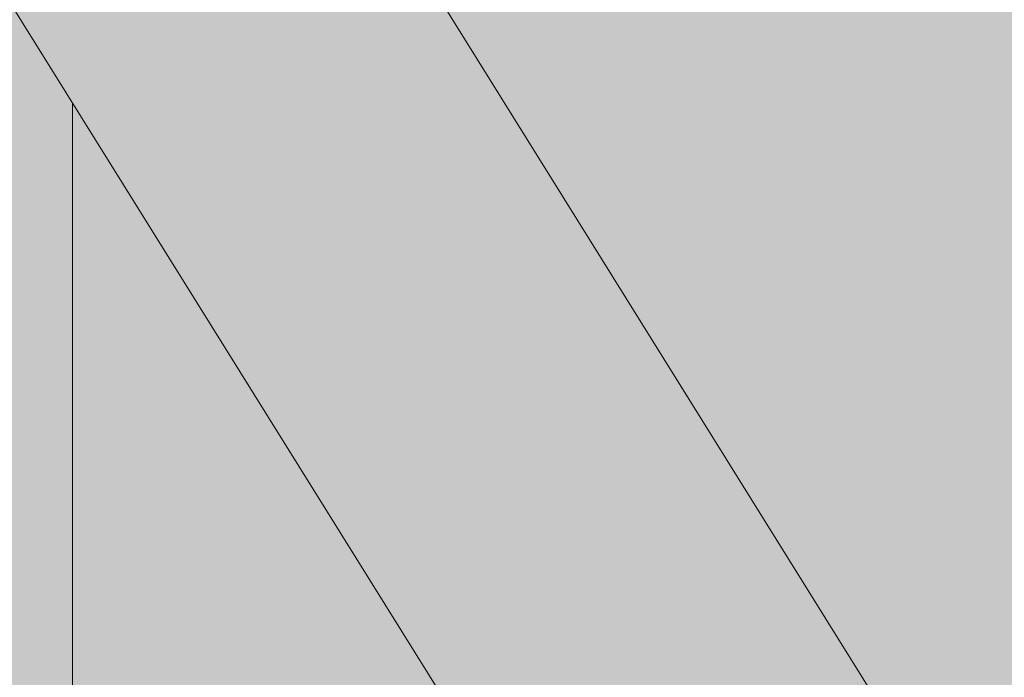
# Model space of a CAD drawing. Units: millimetres. Extents: x 11032 to 26788, y 3406 to 24505.
# Tile 50 of 78: x 15652 to 15786, y 16276 to 16366. Entities that reach past the tile are written whole.
import ezdxf

# ---------------------------------------------------------------- set-up
doc = ezdxf.new("R2010")
doc.units = ezdxf.units.MM
doc.header["$MEASUREMENT"] = 0
for name, color, linetype, lineweight in [('A-ANNO-DIMS', 2, 'Continuous', 18), ('A-GLAZ', 250, 'Continuous', 20), ('A-ROOF', 7, 'Continuous', 30), ('A-WALL', 7, 'Continuous', 35), ('E-LITE', 7, 'Continuous', 18), ('E-LITE-PATT', 7, 'Continuous', 13)]:
    doc.layers.add(name, color=color, linetype=linetype, lineweight=lineweight)
for name, color, linetype, lineweight, true_color in [('A-GLAZ-FRAM-PATT', 250, 'Continuous', 13, 0x262627), ('A-ROOF-PATT', 9, 'Continuous', 13, 0xc7c8ca), ('A-WALL-INTR-PATT', 251, 'Continuous', 13, 0x6c6b6a)]:
    doc.layers.add(name, color=color, linetype=linetype, lineweight=lineweight, true_color=true_color)
doc.styles.get("Standard").update_dxf_attribs({"font": 'arial.ttf'})
doc.dimstyles.get("Standard").update_dxf_attribs({"dimtxt": 150, "dimasz": 100, "dimexe": 10, "dimexo": 5, "dimgap": 5, "dimtad": 0, "dimtih": 1, "dimtoh": 1, "dimdec": 0, "dimzin": 0, "dimdsep": 46, "dimtxsty": 'Standard', "dimcen": 0.09, "dimadec": 0, "dimazin": 0, "dimtfac": 1, "dimtdec": 0, "dimtofl": 0, "dimtmove": 0, "dimatfit": 3, "dimfxl": 1, "dimtolj": 1, "dimtzin": 0, "dimarcsym": 0})

# ---------------------------------------------------------------- blocks, each defined once
blk = doc.blocks.new('*D36')
at = {"layer": 'A-ANNO-DIMS', "color": 0, "lineweight": -2, "transparency": 16777216}
for p, q in [((12301.26, 17115.89), (12301.26, 24416.86)), ((25397.4, 4466.4), (25397.4, 24416.86)), ((12401.26, 24406.86), (18569.2, 24406.86)), ((25297.4, 24406.86), (19129.47, 24406.86))]:
    blk.add_line(p, q, dxfattribs=at)
at = {"layer": 'A-ANNO-DIMS', "color": 0, "transparency": 16777216}
for points in [[(12401.26, 24423.52), (12401.26, 24390.19), (12301.26, 24406.86)], [(25297.4, 24423.52), (25297.4, 24390.19), (25397.4, 24406.86)]]:
    blk.add_solid(points, dxfattribs=at)
at = {"layer": 'Defpoints', "color": 0, "transparency": 16777216}
for p in [(25397.4, 24406.86), (12301.26, 17110.89), (25397.4, 4461.4)]:
    blk.add_point(p, dxfattribs=at)
at = {"layer": 'A-ANNO-DIMS', "color": 0, "transparency": 16777216, "insert": (18849.33, 24406.86), "char_height": 150, "attachment_point": 5}
blk.add_mtext('\\A1;13096', dxfattribs=at)
blk = doc.blocks.new('*D37')
at = {"layer": 'A-ANNO-DIMS', "color": 0, "lineweight": -2, "transparency": 16777216}
for p, q in [((18087.74, 23450.36), (11334.76, 23450.36)), ((11344.76, 23350.36), (11344.76, 14037.46)), ((11344.76, 4561.4), (11344.76, 13874.29)), ((12927.66, 4461.4), (11334.76, 4461.4))]:
    blk.add_line(p, q, dxfattribs=at)
at = {"layer": 'A-ANNO-DIMS', "color": 0, "transparency": 16777216}
for points in [[(11328.1, 23350.36), (11361.43, 23350.36), (11344.76, 23450.36)], [(11328.1, 4561.4), (11361.43, 4561.4), (11344.76, 4461.4)]]:
    blk.add_solid(points, dxfattribs=at)
at = {"layer": 'Defpoints', "color": 0, "transparency": 16777216}
for p in [(11344.76, 23450.36), (18092.74, 23450.36), (12932.66, 4461.4)]:
    blk.add_point(p, dxfattribs=at)
at = {"layer": 'A-ANNO-DIMS', "color": 0, "transparency": 16777216, "insert": (11344.76, 13955.88), "char_height": 150, "attachment_point": 5}
blk.add_mtext('\\A1;18989', dxfattribs=at)
blk = doc.blocks.new('*D45')
at = {"layer": 'A-ANNO-DIMS', "color": 0, "lineweight": -2, "transparency": 16777216}
for p, q in [((13792.37, 18518.92), (26363.9, 18518.92)), ((26353.9, 18418.92), (26353.9, 17450.32)), ((26353.9, 16318.44), (26353.9, 17287.05)), ((22902.4, 16218.44), (26363.9, 16218.44))]:
    blk.add_line(p, q, dxfattribs=at)
at = {"layer": 'A-ANNO-DIMS', "color": 0, "transparency": 16777216}
for points in [[(26337.24, 18418.92), (26370.57, 18418.92), (26353.9, 18518.92)], [(26337.24, 16318.44), (26370.57, 16318.44), (26353.9, 16218.44)]]:
    blk.add_solid(points, dxfattribs=at)
at = {"layer": 'Defpoints', "color": 0, "transparency": 16777216}
for p in [(13787.37, 18518.92), (26353.9, 18518.92), (22897.4, 16218.44)]:
    blk.add_point(p, dxfattribs=at)
at = {"layer": 'A-ANNO-DIMS', "color": 0, "transparency": 16777216, "insert": (26353.9, 17368.68), "char_height": 150, "attachment_point": 5}
blk.add_mtext('\\A1;2300.5', dxfattribs=at)
blk = doc.blocks.new('*D57')
at = {"layer": 'A-ANNO-DIMS', "color": 0, "lineweight": -2, "transparency": 16777216}
for p, q in [((14994.7, 7266.4), (14994.7, 24416.86)), ((20894.7, 7266.4), (20894.7, 24416.86)), ((15094.7, 24406.86), (17715.98, 24406.86)), ((20794.7, 24406.86), (18173.42, 24406.86))]:
    blk.add_line(p, q, dxfattribs=at)
at = {"layer": 'A-ANNO-DIMS', "color": 0, "transparency": 16777216}
for points in [[(15094.7, 24423.52), (15094.7, 24390.19), (14994.7, 24406.86)], [(20794.7, 24423.52), (20794.7, 24390.19), (20894.7, 24406.86)]]:
    blk.add_solid(points, dxfattribs=at)
at = {"layer": 'Defpoints', "color": 0, "transparency": 16777216}
for p in [(20894.7, 24406.86), (14994.7, 7261.4), (20894.7, 7261.4)]:
    blk.add_point(p, dxfattribs=at)
at = {"layer": 'A-ANNO-DIMS', "color": 0, "transparency": 16777216, "insert": (17944.7, 24406.86), "char_height": 150, "attachment_point": 5}
blk.add_mtext('\\A1;5900', dxfattribs=at)
blk = doc.blocks.new('*D60')
at = {"layer": 'A-ANNO-DIMS', "color": 0, "lineweight": -2, "transparency": 16777216}
for p, q in [((14994.7, 7266.4), (14994.7, 24416.86)), ((16344.7, 7266.4), (16344.7, 24416.86)), ((15094.7, 24406.86), (15448.04, 24406.86)), ((16244.7, 24406.86), (15891.36, 24406.86))]:
    blk.add_line(p, q, dxfattribs=at)
at = {"layer": 'A-ANNO-DIMS', "color": 0, "transparency": 16777216}
for points in [[(15094.7, 24423.52), (15094.7, 24390.19), (14994.7, 24406.86)], [(16244.7, 24423.52), (16244.7, 24390.19), (16344.7, 24406.86)]]:
    blk.add_solid(points, dxfattribs=at)
at = {"layer": 'Defpoints', "color": 0, "transparency": 16777216}
for p in [(16344.7, 24406.86), (14994.7, 7261.4), (16344.7, 7261.4)]:
    blk.add_point(p, dxfattribs=at)
at = {"layer": 'A-ANNO-DIMS', "color": 0, "transparency": 16777216, "insert": (15669.7, 24406.86), "char_height": 150, "attachment_point": 5}
blk.add_mtext('\\A1;1350', dxfattribs=at)

msp = doc.modelspace()

# ---------------------------------------------------------------- hatches: boundary and pattern name
at = {"layer": 'A-GLAZ-FRAM-PATT'}
h = msp.add_hatch(color=256, dxfattribs=at)
edge = h.paths.add_edge_path()
edge.add_line((15284.393, 17051.32), (15084.393, 17001.32))
edge.add_line((15084.393, 17001.32), (15084.393, 15951.32))
edge.add_spline(control_points=[(15084.393, 15951.32), (15157.266, 15924.219), (15224.458, 15897.808), (15284.393, 15870.289)], knot_values=[511.9490104, 511.9490104, 511.9490104, 511.9490104, 697.3715979, 697.3715979, 697.3715979, 697.3715979], degree=3, periodic=0)
edge.add_line((15284.393, 15870.289), (15284.393, 17051.32))
edge = h.paths.add_edge_path()
edge.add_line((15659.393, 16354.387), (15459.393, 16675.629))
edge.add_line((15459.393, 16675.629), (15459.393, 15771.505))
edge.add_spline(control_points=[(15459.393, 15771.505), (15501.891, 15741.568), (15571.096, 15682.692), (15632.72, 15612.509), (15659.393, 15578.299)], knot_values=[905.064582, 905.064582, 905.064582, 905.064582, 1079.4682707, 1223.1584353, 1223.1584353, 1223.1584353, 1223.1584353], degree=3, periodic=0)
edge.add_line((15659.393, 15578.299), (15659.393, 16354.387))
h.paths.add_polyline_path([(15284.393, 17051.32), (15284.393, 16956.717), (15784.393, 16153.61), (15784.393, 16248.213)])
at = {"layer": 'A-ROOF-PATT'}
h = msp.add_hatch(color=256, dxfattribs=at)
edge = h.paths.add_edge_path()
edge.add_spline(control_points=[(17532.827, 17324.837), (17391.335, 17349.016), (16840.872, 17494.912), (16080.055, 18069.544), (14738.803, 18299.641), (13382.429, 18838.336), (12580.532, 17870.207), (12430.422, 17563.822)], knot_values=[2977.6027945, 2977.6027945, 2977.6027945, 2977.6027945, 3438.1840601, 4811.6463022, 5622.8675483, 7588.0288188, 8560.6685791, 8560.6685791, 8560.6685791, 8560.6685791], degree=3, periodic=0)
edge.add_spline(control_points=[(12430.422, 17563.822), (12437.904, 17573.36), (12445.386, 17582.899), (12452.869, 17592.437), (12452.869, 17592.438), (12452.869, 17592.438), (12452.869, 17592.438)], knot_values=[1408.564138, 1408.564138, 1408.564138, 1408.564138, 1444.85989, 1444.85989, 1444.85989, 1444.8601183, 1444.8601183, 1444.8601183, 1444.8601183], degree=3, periodic=0)
edge.add_spline(control_points=[(12452.869, 17592.438), (12555.432, 17723.185), (12736.557, 17929.686), (13044.86, 18114.643), (13219.943, 18189.644), (13299.92, 18220.646)], knot_values=[339.318246, 339.318246, 339.318246, 339.318246, 836.8349967, 1151.2512933, 1408.564138, 1408.564138, 1408.564138, 1408.564138], degree=3, periodic=0)
edge.add_spline(control_points=[(13299.92, 18220.646), (13299.998, 18220.689), (13300.077, 18220.732), (13319.738, 18231.488), (13339.24, 18241.402), (13388.645, 18264.703), (13418.466, 18277.069), (13478.019, 18298.648), (13507.751, 18307.861), (13544.561, 18317.488), (13551.584, 18319.245), (13558.612, 18320.924)], knot_values=[3783.8950972, 3783.8950972, 3783.8950972, 3783.8950972, 3784.1737101, 3784.1737101, 3853.4666747, 3853.4666747, 3960.2401917, 3960.2401917, 4067.0137087, 4067.0137087, 4092.1744649, 4092.1744649, 4092.1744649, 4092.1744649], degree=3, periodic=0)
edge.add_spline(control_points=[(13558.612, 18320.924), (13581.407, 18326.373), (13604.25, 18331.007), (13657.184, 18339.957), (13687.338, 18343.732), (13748.098, 18348.892), (13778.704, 18350.276), (13840.46, 18350.833), (13871.609, 18350.005), (13934.496, 18346.313), (13966.232, 18343.449), (14030.297, 18335.871), (14062.625, 18331.158), (14127.853, 18320.088), (14160.753, 18313.73), (14241.357, 18296.556), (14289.343, 18284.997), (14386.31, 18259.688), (14435.291, 18245.941), (14534.161, 18217.034), (14584.049, 18201.875), (14684.682, 18170.964), (14735.427, 18155.212), (14837.763, 18123.971), (14889.354, 18108.482), (14954.971, 18089.677), (14968.586, 18085.823), (14992.391, 18079.184), (15002.566, 18076.376), (15021.739, 18071.153), (15030.731, 18068.729), (15047.707, 18064.21), (15055.694, 18062.106), (15079.815, 18055.825), (15095.905, 18051.728), (15143.966, 18039.717), (15175.729, 18032.084), (15254.84, 18013.501), (15301.798, 18002.866), (15394.186, 17981.845), (15439.615, 17971.459), (15528.833, 17950.135), (15572.62, 17939.197), (15658.477, 17916.021), (15700.546, 17903.785), (15753.633, 17886.734), (15765.446, 17882.835), (15786.574, 17875.653), (15795.915, 17872.404), (15810.108, 17867.349), (15814.99, 17865.588), (15824.736, 17862.029), (15829.611, 17860.226), (15844.241, 17854.75), (15854.002, 17851.008), (15883.312, 17839.521), (15902.885, 17831.512), (15966.355, 17804.548), (16010.39, 17784.302), (16098.838, 17741.267), (16143.25, 17718.478), (16232.497, 17671.098), (16277.332, 17646.507), (16367.515, 17596.295), (16412.862, 17570.676), (16504.202, 17519.209), (16550.194, 17493.362), (16643.009, 17442.263), (16689.831, 17417.011), (16756.517, 17382.472), (16775.937, 17372.58), (16795.455, 17362.84)], knot_values=[4092.1744649, 4092.1744649, 4092.1744649, 4092.1744649, 4173.7872258, 4173.7872258, 4280.5607428, 4280.5607428, 4387.3342598, 4387.3342598, 4494.1077768, 4494.1077768, 4600.8812939, 4600.8812939, 4707.6548109, 4707.6548109, 4814.4283279, 4814.4283279, 4967.1262405, 4967.1262405, 5119.8241531, 5119.8241531, 5272.5220657, 5272.5220657, 5425.2199783, 5425.2199783, 5577.9178908, 5577.9178908, 5617.7853319, 5617.7853319, 5647.4648479, 5647.4648479, 5673.611025, 5673.611025, 5696.747607, 5696.747607, 5743.6818903, 5743.6818903, 5837.5504571, 5837.5504571, 5979.7261046, 5979.7261046, 6121.9017521, 6121.9017521, 6264.0773996, 6264.0773996, 6406.2530471, 6406.2530471, 6447.2585849, 6447.2585849, 6480.0420882, 6480.0420882, 6497.3077062, 6497.3077062, 6514.5733242, 6514.5733242, 6549.1045602, 6549.1045602, 6618.1670322, 6618.1670322, 6772.6610171, 6772.6610171, 6927.155002, 6927.155002, 7081.6489869, 7081.6489869, 7236.1429718, 7236.1429718, 7390.6369567, 7390.6369567, 7545.1309416, 7545.1309416, 7608.1992868, 7608.1992868, 7608.1992868, 7608.1992868], degree=3, periodic=0)
edge.add_spline(control_points=[(16795.455, 17362.84), (16814.335, 17349.456), (16832.897, 17336.263), (16873.225, 17307.197), (16894.778, 17291.386), (16936.221, 17259.941), (16956.11, 17244.308), (16993.863, 17213.094), (17011.726, 17197.514), (17041.993, 17169.265), (17054.791, 17156.601), (17078.762, 17131.225), (17089.933, 17118.516), (17110.618, 17092.991), (17120.131, 17080.178), (17130.17, 17065.264), (17131.487, 17063.277), (17133.77, 17059.776), (17134.746, 17058.261), (17136.69, 17055.205), (17137.657, 17053.668), (17140.539, 17049.025), (17142.438, 17045.89), (17148.068, 17036.367), (17151.732, 17029.859), (17163.03, 17008.788), (17170.335, 16993.646), (17184.087, 16961.978), (17190.534, 16945.453), (17202.562, 16911.165), (17208.142, 16893.402), (17218.448, 16856.821), (17223.173, 16838.003), (17231.801, 16799.51), (17235.705, 16779.837), (17241.533, 16746.739), (17243.676, 16733.5), (17247.718, 16706.37), (17249.608, 16692.472), (17252.066, 16672.69), (17252.761, 16666.875), (17254.1, 16655.226), (17254.744, 16649.4), (17256.596, 16631.917), (17257.727, 16620.254), (17260.823, 16585.238), (17262.489, 16561.858), (17266.551, 16488.654), (17267.658, 16438.661), (17267.349, 16375.228), (17267.193, 16362.07), (17266.95, 16348.891)], knot_values=[15.1130472, 15.1130472, 15.1130472, 15.1130472, 82.6995146, 82.6995146, 165.3990291, 165.3990291, 248.0985437, 248.0985437, 330.7980583, 330.7980583, 397.9419458, 397.9419458, 465.0858333, 465.0858333, 532.2297209, 532.2297209, 542.533741, 542.533741, 550.3568158, 550.3568158, 558.1798906, 558.1798906, 573.8260402, 573.8260402, 605.1183395, 605.1183395, 672.7640614, 672.7640614, 740.4097834, 740.4097834, 808.0555054, 808.0555054, 875.7012273, 875.7012273, 943.3469493, 943.3469493, 987.6613492, 987.6613492, 1033.4121612, 1033.4121612, 1052.3850876, 1052.3850876, 1071.358014, 1071.358014, 1109.3038668, 1109.3038668, 1185.1955724, 1185.1955724, 1346.4419026, 1346.4419026, 1388.5586631, 1388.5586631, 1388.5586631, 1388.5586631], degree=3, periodic=0)
edge.add_spline(control_points=[(17266.95, 16348.891), (17266.95, 16348.891), (17266.95, 16348.891), (17266.95, 16348.891), (17253.182, 15602.417), (17239.414, 14855.943), (17225.646, 14109.469)], knot_values=[1388.5586631, 1388.5586631, 1388.5586631, 1388.5586631, 1388.5589654, 1388.5589654, 1388.5589654, 3774.0767661, 3774.0767661, 3774.0767661, 3774.0767661], degree=3, periodic=0)
edge.add_spline(control_points=[(17225.646, 14109.469), (17226.198, 14109.827), (17226.748, 14110.185), (17242.065, 14120.191), (17255.956, 14130.116), (17274.422, 14144.286), (17279.609, 14148.386), (17284.686, 14152.511)], knot_values=[1926.3423968, 1926.3423968, 1926.3423968, 1926.3423968, 1927.316729, 1927.316729, 1953.5121761, 1953.5121761, 1964.0732348, 1964.0732348, 1964.0732348, 1964.0732348], degree=3, periodic=0)
edge.add_spline(control_points=[(17284.686, 14152.511), (17315.791, 14194.761), (17384.413, 14446.273), (17407.128, 14793.401), (17407.093, 15295.84), (17423.274, 15626.362), (17415.601, 15782.507)], knot_values=[0, 0, 0, 0, 163.2554674, 619.2296767, 1171.8624483, 1621.6355562, 1621.6355562, 1621.6355562, 1621.6355562], degree=3, periodic=0)
edge.add_spline(control_points=[(17415.601, 15782.507), (17438.21, 16077.57), (17410.495, 16533.484), (17390.893, 17030.649), (17301.082, 17169.349)], knot_values=[543.9784753, 543.9784753, 543.9784753, 543.9784753, 1452.9852767, 1960.0114926, 1960.0114926, 1960.0114926, 1960.0114926], degree=3, periodic=0)
edge.add_spline(control_points=[(17301.082, 17169.349), (17346.58, 17157.64), (17392.235, 17147.336), (17467.161, 17132.609), (17496.336, 17127.412), (17525.58, 17122.709)], knot_values=[8131.593939, 8131.593939, 8131.593939, 8131.593939, 8269.7349273, 8269.7349273, 8357.5016646, 8357.5016646, 8357.5016646, 8357.5016646], degree=3, periodic=0)
edge.add_line((17525.58, 17122.709), (17532.827, 17324.837))
edge = h.paths.add_edge_path(flags=17)
edge.add_spline(control_points=[(13340.537, 14602.706), (13316.172, 14726.456), (13323.666, 14932.342), (13637.836, 15081.117), (13863.248, 15171.051), (14002.1, 15224.503), (14058.539, 15244.876)], knot_values=[680.8931862, 680.8931862, 680.8931862, 680.8931862, 1033.4728289, 1337.4008326, 1604.7214264, 1784.2944722, 1784.2944722, 1784.2944722, 1784.2944722], degree=3, periodic=0)
edge.add_spline(control_points=[(14058.539, 15244.876), (14058.289, 15275.236), (14057.634, 15305.434), (14055.312, 15376.527), (14053.359, 15417.248), (14048.642, 15497.048), (14045.89, 15536.143), (14042.888, 15574.619)], knot_values=[6573.1065419, 6573.1065419, 6573.1065419, 6573.1065419, 6636.7330012, 6636.7330012, 6723.8890547, 6723.8890547, 6809.6328771, 6809.6328771, 6809.6328771, 6809.6328771], degree=3, periodic=0)
edge.add_spline(control_points=[(14042.888, 15574.619), (13546.54, 15403.221), (13074.735, 15143.241), (13277.36, 14695.339), (13340.537, 14602.706)], knot_values=[503.7925783, 503.7925783, 503.7925783, 503.7925783, 1728.1787606, 2051.34844, 2051.34844, 2051.34844, 2051.34844], degree=3, periodic=0)
h = msp.add_hatch(color=256, dxfattribs=at)
h.set_gradient(color1=(254, 234, 185), color2=(254, 204, 102), name='HEMISPHERICAL')
edge = h.paths.add_edge_path()
edge.add_line((15084.393, 17001.32), (15284.393, 17051.32))
edge.add_line((15284.393, 17051.32), (15470.537, 16752.334))
edge.add_spline(control_points=[(15470.537, 16752.334), (15683.311, 16831.508), (16106.827, 16912.335), (16625.609, 16876.997), (17083.498, 16357.78), (17257.801, 16180.113)], knot_values=[0, 0, 0, 0, 655.2936334, 1252.0157838, 1989.6162859, 1989.6162859, 1989.6162859, 1989.6162859], degree=3, periodic=0)
edge.add_spline(control_points=[(17257.801, 16180.113), (17260.851, 16236.372), (17263.9, 16292.632), (17266.95, 16348.891)], knot_values=[1132.9967717, 1132.9967717, 1132.9967717, 1132.9967717, 1198.0464225, 1198.0464225, 1198.0464225, 1198.0464225], degree=3, periodic=0)
edge.add_spline(control_points=[(17266.95, 16348.891), (17267.193, 16362.07), (17267.349, 16375.228), (17267.658, 16438.661), (17266.551, 16488.654), (17262.489, 16561.858), (17260.823, 16585.238), (17257.727, 16620.254), (17256.596, 16631.917), (17254.744, 16649.4), (17254.1, 16655.226), (17252.761, 16666.875), (17252.066, 16672.69), (17249.608, 16692.472), (17247.718, 16706.37), (17243.676, 16733.5), (17241.533, 16746.739), (17235.705, 16779.837), (17231.801, 16799.51), (17223.173, 16838.003), (17218.448, 16856.821), (17208.142, 16893.402), (17202.562, 16911.165), (17190.534, 16945.453), (17184.087, 16961.978), (17170.335, 16993.646), (17163.03, 17008.788), (17151.732, 17029.859), (17148.068, 17036.367), (17142.438, 17045.89), (17140.539, 17049.025), (17137.657, 17053.668), (17136.69, 17055.205), (17134.746, 17058.261), (17133.77, 17059.776), (17131.487, 17063.277), (17130.17, 17065.264), (17120.131, 17080.178), (17110.618, 17092.991), (17089.933, 17118.516), (17078.762, 17131.225), (17054.791, 17156.601), (17041.993, 17169.265), (17011.726, 17197.514), (16993.863, 17213.094), (16956.11, 17244.308), (16936.221, 17259.941), (16894.778, 17291.386), (16873.225, 17307.197), (16832.897, 17336.263), (16814.335, 17349.456), (16795.455, 17362.84)], knot_values=[15.1130472, 15.1130472, 15.1130472, 15.1130472, 57.2298077, 57.2298077, 218.4761379, 218.4761379, 294.3678435, 294.3678435, 332.3136963, 332.3136963, 351.2866227, 351.2866227, 370.2595491, 370.2595491, 416.0103612, 416.0103612, 460.324761, 460.324761, 527.970483, 527.970483, 595.616205, 595.616205, 663.2619269, 663.2619269, 730.9076489, 730.9076489, 798.5533709, 798.5533709, 829.8456701, 829.8456701, 845.4918197, 845.4918197, 853.3148945, 853.3148945, 861.1379693, 861.1379693, 871.4419895, 871.4419895, 938.585877, 938.585877, 1005.7297645, 1005.7297645, 1072.8736521, 1072.8736521, 1155.5731666, 1155.5731666, 1238.2726812, 1238.2726812, 1320.9721958, 1320.9721958, 1388.5586631, 1388.5586631, 1388.5586631, 1388.5586631], degree=3, periodic=0)
edge.add_spline(control_points=[(16795.455, 17362.84), (16775.937, 17372.58), (16756.517, 17382.472), (16689.831, 17417.011), (16643.009, 17442.263), (16550.194, 17493.362), (16504.202, 17519.209), (16412.862, 17570.676), (16367.515, 17596.295), (16277.332, 17646.507), (16232.497, 17671.098), (16143.25, 17718.478), (16098.838, 17741.267), (16010.39, 17784.302), (15966.355, 17804.548), (15902.885, 17831.512), (15883.312, 17839.521), (15854.002, 17851.008), (15844.241, 17854.75), (15829.611, 17860.226), (15824.736, 17862.029), (15814.99, 17865.588), (15810.108, 17867.349), (15795.915, 17872.404), (15786.574, 17875.653), (15765.446, 17882.835), (15753.633, 17886.734), (15700.546, 17903.785), (15658.477, 17916.021), (15572.62, 17939.197), (15528.833, 17950.135), (15439.615, 17971.459), (15394.186, 17981.845), (15301.798, 18002.866), (15254.84, 18013.501), (15175.729, 18032.084), (15143.966, 18039.717), (15095.905, 18051.728), (15079.815, 18055.825), (15055.694, 18062.106), (15047.707, 18064.21), (15030.731, 18068.729), (15021.739, 18071.153), (15002.566, 18076.376), (14992.391, 18079.184), (14968.586, 18085.823), (14954.971, 18089.677), (14889.354, 18108.482), (14837.763, 18123.971), (14735.427, 18155.212), (14684.682, 18170.964), (14584.049, 18201.875), (14534.161, 18217.034), (14435.291, 18245.941), (14386.31, 18259.688), (14289.343, 18284.997), (14241.357, 18296.556), (14160.753, 18313.73), (14127.853, 18320.088), (14062.625, 18331.158), (14030.297, 18335.871), (13966.232, 18343.449), (13934.496, 18346.313), (13871.609, 18350.005), (13840.46, 18350.833), (13778.704, 18350.276), (13748.098, 18348.892), (13687.338, 18343.732), (13657.184, 18339.957), (13604.25, 18331.007), (13581.407, 18326.373), (13558.612, 18320.924)], knot_values=[4092.1744649, 4092.1744649, 4092.1744649, 4092.1744649, 4155.2428101, 4155.2428101, 4309.736795, 4309.736795, 4464.2307799, 4464.2307799, 4618.7247648, 4618.7247648, 4773.2187497, 4773.2187497, 4927.7127346, 4927.7127346, 5082.2067195, 5082.2067195, 5151.2691915, 5151.2691915, 5185.8004275, 5185.8004275, 5203.0660455, 5203.0660455, 5220.3316635, 5220.3316635, 5253.1151668, 5253.1151668, 5294.1207046, 5294.1207046, 5436.2963521, 5436.2963521, 5578.4719996, 5578.4719996, 5720.6476471, 5720.6476471, 5862.8232946, 5862.8232946, 5956.6918614, 5956.6918614, 6003.6261447, 6003.6261447, 6026.7627267, 6026.7627267, 6052.9089038, 6052.9089038, 6082.5884198, 6082.5884198, 6122.4558609, 6122.4558609, 6275.1537734, 6275.1537734, 6427.851686, 6427.851686, 6580.5495986, 6580.5495986, 6733.2475112, 6733.2475112, 6885.9454238, 6885.9454238, 6992.7189408, 6992.7189408, 7099.4924578, 7099.4924578, 7206.2659749, 7206.2659749, 7313.0394919, 7313.0394919, 7419.8130089, 7419.8130089, 7526.5865259, 7526.5865259, 7608.1992868, 7608.1992868, 7608.1992868, 7608.1992868], degree=3, periodic=0)
edge.add_spline(control_points=[(13558.612, 18320.924), (13472.381, 18287.498), (13386.15, 18254.072), (13299.92, 18220.646), (13299.92, 18220.646), (13299.92, 18220.646), (13299.92, 18220.646)], knot_values=[61.8832457, 61.8832457, 61.8832457, 61.8832457, 339.3179746, 339.3179746, 339.3179746, 339.318246, 339.318246, 339.318246, 339.318246], degree=3, periodic=0)
edge.add_spline(control_points=[(13299.92, 18220.646), (13219.943, 18189.644), (13044.86, 18114.643), (12736.557, 17929.686), (12555.432, 17723.185), (12452.869, 17592.438)], knot_values=[339.318246, 339.318246, 339.318246, 339.318246, 596.6310906, 911.0473872, 1408.564138, 1408.564138, 1408.564138, 1408.564138], degree=3, periodic=0)
edge.add_spline(control_points=[(12452.869, 17592.438), (12452.869, 17592.438), (12452.869, 17592.438), (12452.869, 17592.437), (12445.386, 17582.899), (12437.904, 17573.36), (12430.422, 17563.822)], knot_values=[1408.564138, 1408.564138, 1408.564138, 1408.564138, 1408.5643663, 1408.5643663, 1408.5643663, 1444.8601183, 1444.8601183, 1444.8601183, 1444.8601183], degree=3, periodic=0)
edge.add_spline(control_points=[(12430.422, 17563.822), (12373.797, 17448.248), (12157.302, 16836.764), (12751.985, 16393.69), (13424.325, 15907.903), (14042.888, 15574.619)], knot_values=[0, 0, 0, 0, 366.8993034, 1975.5941082, 2977.6027945, 2977.6027945, 2977.6027945, 2977.6027945], degree=3, periodic=0)
edge.add_spline(control_points=[(14042.888, 15574.619), (14042.839, 15575.252), (14042.789, 15575.886), (14039.681, 15615.607), (14036.366, 15654.052), (14029.551, 15729.305), (14026.05, 15766.114), (14019.175, 15837.686), (14015.8, 15872.45), (13903.823, 16338.596)], knot_values=[6310.2261504, 6310.2261504, 6310.2261504, 6310.2261504, 6311.6383814, 6311.6383814, 6398.7944349, 6398.7944349, 6485.9504884, 6485.9504884, 6573.1065419, 6573.1065419, 6573.1065419, 6573.1065419], degree=3, periodic=0)
edge.add_spline(control_points=[(13903.823, 16338.596), (14237.315, 16236.889), (14456.623, 16167.555), (14614.196, 16115.84)], knot_values=[0, 0, 0, 0, 202.9853419, 202.9853419, 202.9853419, 202.9853419], degree=3, periodic=0)
edge.add_spline(control_points=[(14614.196, 16115.84), (14663.209, 16178.992), (14799.965, 16341.237), (14969.915, 16481.426), (15084.393, 16556.825)], knot_values=[2405.0345045, 2405.0345045, 2405.0345045, 2405.0345045, 2644.8826966, 3039.2707272, 3039.2707272, 3039.2707272, 3039.2707272], degree=3, periodic=0)
edge.add_line((15084.393, 16556.825), (15084.393, 17001.32))
h.paths.add_polyline_path([(14195.599, 17606.181, -1), (14395.599, 17606.181, -1)], flags=16)
h.paths.add_polyline_path([(13310.178, 17032.97, -1), (13510.178, 17032.97, -1)], flags=16)
h = msp.add_hatch(color=256, dxfattribs=at)
h.set_gradient(color1=(254, 234, 185), color2=(254, 204, 102), name='HEMISPHERICAL')
edge = h.paths.add_edge_path()
edge.add_spline(control_points=[(16560.042, 14907.752), (16569.192, 14907.664), (16578.343, 14907.575), (16587.493, 14907.486), (16832.101, 14905.115), (17122.895, 14902.296), (16849.359, 14976.117), (16870.954, 15304.114), (17098.337, 15241.178), (17235.385, 15203.245)], knot_values=[0, 0, 0, 0, 14.8674385, 14.8674385, 14.8674385, 412.2943091, 487.3345915, 708.6416004, 1044.3939449, 1044.3939449, 1044.3939449, 1044.3939449], degree=3, periodic=0)
edge.add_line((16587.504, 14907.486), (16560.207, 14907.486))
edge.add_line((16560.207, 14907.486), (15784.393, 16153.61))
edge.add_line((15784.393, 16153.61), (15784.393, 15385.996))
edge.add_spline(control_points=[(15784.393, 15385.996), (15798.391, 15360.52), (15847.198, 15266.214), (15887.196, 15168.614), (15912.903, 15096.727)], knot_values=[1463.2850479, 1463.2850479, 1463.2850479, 1463.2850479, 1550.659771, 1779.9599361, 1779.9599361, 1779.9599361, 1779.9599361], degree=3, periodic=0)
edge.add_spline(control_points=[(15912.903, 15096.727), (15913.652, 15095.649), (15914.403, 15094.565), (15925.191, 15078.948), (15935.516, 15063.47), (15956.582, 15030.918), (15967.324, 15013.844), (15989.119, 14978.386), (16000.173, 14960.003), (16022.525, 14922.193), (16033.824, 14902.767), (16056.63, 14863.116), (16068.138, 14842.891), (16091.349, 14801.871), (16103.053, 14781.075), (16126.666, 14739.118), (16138.575, 14717.958), (16162.628, 14675.459), (16174.772, 14654.12), (16199.352, 14611.428), (16211.787, 14590.075), (16237.037, 14547.491), (16249.851, 14526.26), (16271.946, 14490.566), (16281.092, 14476.044), (16299.694, 14447.129), (16309.149, 14432.737), (16328.456, 14404.098), (16338.307, 14389.85), (16358.518, 14361.503), (16368.879, 14347.403), (16390.266, 14319.347), (16401.291, 14305.391), (16420.626, 14281.969), (16428.703, 14272.467), (16445.363, 14253.527), (16453.946, 14244.088), (16471.727, 14225.278), (16480.926, 14215.907), (16500.075, 14197.247), (16510.026, 14187.959), (16530.844, 14169.504), (16541.71, 14160.337), (16564.549, 14142.195), (16576.522, 14133.22), (16597.69, 14118.448), (16606.528, 14112.565), (16624.87, 14101.004), (16634.376, 14095.326), (16654.117, 14084.255), (16664.352, 14078.862), (16685.603, 14068.46), (16696.619, 14063.452), (16719.46, 14053.944), (16731.285, 14049.444), (16755.742, 14041.097), (16768.374, 14037.251), (16794.396, 14030.368), (16807.787, 14027.332), (16835.229, 14022.23), (16849.279, 14020.163), (16877.882, 14017.141), (16892.435, 14016.186), (16921.835, 14015.489), (16936.683, 14015.749), (16961.564, 14017.241), (16971.582, 14018.127), (16986.57, 14019.883), (16991.56, 14020.54), (16999.027, 14021.63), (17001.514, 14022.011), (17006.48, 14022.809), (17008.962, 14023.225), (17014.824, 14024.251), (17018.193, 14024.875), (17036.262, 14028.398), (17050.55, 14031.826), (17078.171, 14039.583), (17091.505, 14043.912), (17115.643, 14052.705), (17126.557, 14057.089), (17137.108, 14061.688)], knot_values=[2010.7639617, 2010.7639617, 2010.7639617, 2010.7639617, 2014.7029827, 2014.7029827, 2067.238337, 2067.238337, 2119.7736913, 2119.7736913, 2172.3090457, 2172.3090457, 2224.8444, 2224.8444, 2277.3797543, 2277.3797543, 2329.9151086, 2329.9151086, 2382.450463, 2382.450463, 2434.9858173, 2434.9858173, 2487.5211716, 2487.5211716, 2540.0565259, 2540.0565259, 2576.3179289, 2576.3179289, 2612.5793318, 2612.5793318, 2648.8407347, 2648.8407347, 2685.1021376, 2685.1021376, 2721.3635405, 2721.3635405, 2746.252015, 2746.252015, 2771.1404895, 2771.1404895, 2796.028964, 2796.028964, 2820.9174385, 2820.9174385, 2845.8059131, 2845.8059131, 2870.6943876, 2870.6943876, 2887.5132757, 2887.5132757, 2904.3321639, 2904.3321639, 2921.1510521, 2921.1510521, 2937.9699402, 2937.9699402, 2954.7888284, 2954.7888284, 2971.6077166, 2971.6077166, 2988.4266047, 2988.4266047, 3005.2454929, 3005.2454929, 3022.0643811, 3022.0643811, 3038.8832692, 3038.8832692, 3050.1975453, 3050.1975453, 3055.8546833, 3055.8546833, 3058.6832524, 3058.6832524, 3061.5118214, 3061.5118214, 3065.3934173, 3065.3934173, 3082.4668716, 3082.4668716, 3099.5403259, 3099.5403259, 3114.5433443, 3114.5433443, 3114.5433443, 3114.5433443], degree=3, periodic=0)
edge.add_spline(control_points=[(17137.108, 14061.688), (17165.253, 14274.398), (17209.97, 14653.885), (17230.2, 15035.586), (17235.385, 15203.245)], knot_values=[1968.0804557, 1968.0804557, 1968.0804557, 1968.0804557, 2611.5282875, 3114.5379264, 3114.5379264, 3114.5379264, 3114.5379264], degree=3, periodic=0)
edge = h.paths.add_edge_path()
edge.add_spline(control_points=[(16856.103, 14956.992), (16852.841, 14961.219), (16849.83, 14965.576), (16842.539, 14977.287), (16838.658, 14984.798), (16832.033, 15000.109), (16829.289, 15007.911), (16824.126, 15026.008), (16822.047, 15036.354), (16819.308, 15057.097), (16818.649, 15067.496), (16818.576, 15088.188), (16819.162, 15098.483), (16821.467, 15118.823), (16823.186, 15128.868), (16827.696, 15148.567), (16830.486, 15158.22), (16836.065, 15173.969), (16838.565, 15180.211), (16844.079, 15192.402), (16847.092, 15198.353), (16852.029, 15207.021), (16853.744, 15209.868), (16857.321, 15215.468), (16859.188, 15218.226), (16863.017, 15223.558), (16864.978, 15226.136), (16872.565, 15235.558), (16878.593, 15241.952), (16891.428, 15253.591), (16898.232, 15258.834), (16912.397, 15268.127), (16919.756, 15272.176), (16934.816, 15279.138), (16942.515, 15282.052), (16958.1, 15286.873), (16965.985, 15288.78), (16984.013, 15292.142), (16994.186, 15293.334), (17014.631, 15294.619), (17024.904, 15294.713), (17048.453, 15293.935), (17061.76, 15292.783), (17088.519, 15289.422), (17101.972, 15287.211), (17131.961, 15281.46), (17148.526, 15277.734), (17181.692, 15269.627), (17198.292, 15265.245), (17222.182, 15258.759), (17229.535, 15256.737), (17236.862, 15254.714)], knot_values=[9.6639535, 9.6639535, 9.6639535, 9.6639535, 20.0351668, 20.0351668, 36.9411752, 36.9411752, 53.8471837, 53.8471837, 75.7795687, 75.7795687, 97.7119538, 97.7119538, 119.6443388, 119.6443388, 141.5767238, 141.5767238, 163.5091089, 163.5091089, 178.3829945, 178.3829945, 193.2568801, 193.2568801, 200.6938229, 200.6938229, 208.1307657, 208.1307657, 215.4448585, 215.4448585, 235.5795923, 235.5795923, 255.7143261, 255.7143261, 275.8490598, 275.8490598, 295.9837936, 295.9837936, 316.1185274, 316.1185274, 341.7220543, 341.7220543, 367.3255812, 367.3255812, 400.1572431, 400.1572431, 432.988905, 432.988905, 473.0440165, 473.0440165, 513.099128, 513.099128, 530.9692999, 530.9692999, 530.9692999, 530.9692999], degree=3, periodic=0)
edge.add_spline(control_points=[(17236.862, 15254.714), (17240.377, 15387.456), (17242.496, 15609.536), (17239.752, 15831.567), (17250.544, 16044.717)], knot_values=[1250.9818616, 1250.9818616, 1250.9818616, 1250.9818616, 1649.1516581, 1916.613987, 1916.613987, 1916.613987, 1916.613987], degree=3, periodic=0)
edge.add_spline(control_points=[(17250.544, 16044.717), (17229.169, 16066.505), (17207.794, 16088.292), (17186.419, 16110.08), (17186.418, 16110.08), (17186.418, 16110.081), (17186.418, 16110.081)], knot_values=[-88.5185581, -88.5185581, -88.5185581, -88.5185581, -0.0012784, -0.0012784, -0.0012784, 0, 0, 0, 0], degree=3, periodic=0)
edge.add_spline(control_points=[(17186.418, 16110.081), (17169.261, 16127.569), (17151.499, 16145.947), (17114.892, 16184.084), (17096.046, 16203.842), (17057.437, 16244.305), (17037.673, 16265.01), (16997.415, 16306.918), (16976.921, 16328.12), (16927.79, 16378.347), (16898.924, 16407.388), (16840.771, 16464.327), (16811.484, 16492.225), (16758.449, 16540.764), (16734.666, 16561.798), (16687.634, 16601.588), (16664.382, 16620.344), (16624.116, 16650.909), (16606.897, 16663.324), (16583.769, 16678.999), (16577.49, 16683.149), (16567.144, 16689.805), (16563.039, 16692.397), (16550.823, 16699.959), (16542.775, 16704.739), (16526.841, 16713.814), (16518.956, 16718.108), (16495.524, 16730.301), (16480.199, 16737.514), (16449.97, 16750.334), (16435.066, 16755.942), (16405.476, 16765.764), (16390.79, 16769.979), (16361.418, 16777.195), (16346.731, 16780.197), (16317.147, 16785.133), (16302.249, 16787.067), (16272.053, 16789.992), (16256.756, 16790.981), (16225.609, 16792.125), (16209.759, 16792.279), (16177.385, 16791.865), (16160.862, 16791.296), (16136.98, 16790.07), (16129.942, 16789.661), (16118.22, 16788.91), (16113.574, 16788.594), (16103.645, 16787.886), (16098.362, 16787.489), (16087.761, 16786.652), (16082.439, 16786.212), (16066.413, 16784.825), (16055.649, 16783.812), (16023.135, 16780.505), (16001.164, 16777.942), (15934.539, 16769.141), (15889.17, 16761.791), (15797.417, 16743.949), (15751.033, 16733.457), (15645.217, 16705.796), (15585.74, 16687.58), (15526.207, 16666.217), (15525.367, 16665.915), (15524.528, 16665.613)], knot_values=[0, 0, 0, 0, 71.0501454, 71.0501454, 142.1002909, 142.1002909, 213.1504363, 213.1504363, 284.2005818, 284.2005818, 381.323193, 381.323193, 478.4458043, 478.4458043, 557.8219847, 557.8219847, 637.1981651, 637.1981651, 698.3122593, 698.3122593, 721.3971375, 721.3971375, 736.7790891, 736.7790891, 767.5429924, 767.5429924, 798.3068957, 798.3068957, 859.8347022, 859.8347022, 921.3625088, 921.3625088, 982.8903154, 982.8903154, 1044.4181219, 1044.4181219, 1105.9459285, 1105.9459285, 1167.4737351, 1167.4737351, 1229.0015416, 1229.0015416, 1290.5293482, 1290.5293482, 1315.8990035, 1315.8990035, 1332.3812792, 1332.3812792, 1350.9052657, 1350.9052657, 1369.4292522, 1369.4292522, 1406.4772252, 1406.4772252, 1480.5731712, 1480.5731712, 1628.7650633, 1628.7650633, 1776.9569554, 1776.9569554, 1966.3109251, 1966.3109251, 1969.019495, 1969.019495, 1969.019495, 1969.019495], degree=3, periodic=0)
edge.add_line((15524.528, 16665.613), (16587.978, 14957.484))
edge.add_spline(control_points=[(16587.978, 14957.484), (16605.253, 14957.316), (16622.516, 14957.149), (16665.945, 14956.759), (16691.933, 14956.554), (16742.419, 14956.302), (16766.918, 14956.255), (16813.531, 14956.412), (16835.647, 14956.617), (16856.103, 14956.992)], knot_values=[872.2181925, 872.2181925, 872.2181925, 872.2181925, 900.2857301, 900.2857301, 943.3659889, 943.3659889, 986.4462476, 986.4462476, 1029.5265064, 1029.5265064, 1029.5265064, 1029.5265064], degree=3, periodic=0)
h.paths.add_polyline_path([(16474.605, 15622.642, -1), (16624.605, 15622.642, -1)], flags=16)
h.paths.add_polyline_path([(16198.536, 16037.613, -1), (16348.536, 16037.613, -1)], flags=16)
h.paths.add_polyline_path([(16475.717, 16408.125, -1), (16625.717, 16408.125, -1)], flags=16)
at = {"layer": 'A-WALL-INTR-PATT'}
h = msp.add_hatch(color=256, dxfattribs=at)
edge = h.paths.add_edge_path()
edge.add_line((15334.393, 16876.406), (15284.393, 16956.717))
edge.add_line((15284.393, 16956.717), (15284.393, 15870.289))
edge.add_spline(control_points=[(15284.393, 15870.289), (15297.64, 15864.208), (15314.459, 15856.202), (15330.647, 15848.071), (15334.393, 15846.165)], knot_values=[697.3715979, 697.3715979, 697.3715979, 697.3715979, 738.3518582, 750.8383504, 750.8383504, 750.8383504, 750.8383504], degree=3, periodic=0)
edge.add_line((15334.393, 15846.165), (15334.393, 16876.406))
edge = h.paths.add_edge_path()
edge.add_line((15459.393, 16675.629), (15423.061, 16733.987))
edge.add_spline(control_points=[(15423.061, 16733.987), (15418.499, 16732.158), (15413.944, 16730.311), (15409.393, 16728.446)], knot_values=[2038.5222542, 2038.5222542, 2038.5222542, 2038.5222542, 2052.6714029, 2052.6714029, 2052.6714029, 2052.6714029], degree=3, periodic=0)
edge.add_line((15409.393, 16728.446), (15409.393, 15804.345))
edge.add_spline(control_points=[(15409.393, 15804.345), (15426.785, 15793.692), (15443.411, 15782.764), (15459.393, 15771.505)], knot_values=[839.4758736, 839.4758736, 839.4758736, 839.4758736, 905.064582, 905.064582, 905.064582, 905.064582], degree=3, periodic=0)
edge.add_line((15459.393, 15771.505), (15459.393, 16675.629))
edge = h.paths.add_edge_path()
edge.add_line((15709.393, 16274.076), (15659.393, 16354.387))
edge.add_line((15659.393, 16354.387), (15659.393, 15578.299))
edge.add_spline(control_points=[(15659.393, 15578.299), (15676.505, 15556.352), (15693.138, 15533.373), (15709.393, 15509.31)], knot_values=[1223.1584353, 1223.1584353, 1223.1584353, 1223.1584353, 1315.3424293, 1315.3424293, 1315.3424293, 1315.3424293], degree=3, periodic=0)
edge.add_line((15709.393, 15509.31), (15709.393, 16274.076))
at = {"layer": 'E-LITE-PATT'}
h = msp.add_hatch(color=256, dxfattribs=at)
edge = h.paths.add_edge_path()
edge.add_spline(control_points=[(15084.393, 16556.825), (14969.915, 16481.426), (14799.965, 16341.237), (14663.209, 16178.992), (14614.196, 16115.84)], knot_values=[2405.0345045, 2405.0345045, 2405.0345045, 2405.0345045, 2799.422535, 3039.2707272, 3039.2707272, 3039.2707272, 3039.2707272], degree=3, periodic=0)
edge.add_spline(control_points=[(14614.196, 16115.84), (14650.957, 16103.776), (14684.357, 16092.67), (14715.064, 16082.336)], knot_values=[202.9853419, 202.9853419, 202.9853419, 202.9853419, 250.3408615, 250.3408615, 250.3408615, 250.3408615], degree=3, periodic=0)
edge.add_spline(control_points=[(14715.064, 16082.336), (14732.32, 16103.979), (14749.873, 16125.274), (14780.086, 16160.475), (14792.544, 16174.592), (14817.876, 16202.424), (14830.748, 16216.137), (14853.903, 16239.975), (14864.109, 16250.213), (14884.415, 16270.066), (14894.503, 16279.688), (14918.667, 16302.183), (14932.865, 16314.967), (14987.375, 16362.454), (15029.339, 16395.81), (15076.718, 16430.13), (15080.55, 16432.882), (15084.393, 16435.621)], knot_values=[2472.5855096, 2472.5855096, 2472.5855096, 2472.5855096, 2558.786533, 2558.786533, 2617.7975153, 2617.7975153, 2676.8084975, 2676.8084975, 2721.9976237, 2721.9976237, 2765.3424393, 2765.3424393, 2824.4059302, 2824.4059302, 2988.2351723, 2988.2351723, 3002.5987883, 3002.5987883, 3002.5987883, 3002.5987883], degree=3, periodic=0)
edge.add_line((15084.393, 16435.621), (15084.393, 16556.825))
edge = h.paths.add_edge_path()
edge.add_spline(control_points=[(17257.801, 16180.113), (17083.498, 16357.78), (16625.609, 16876.997), (16106.827, 16912.335), (15683.311, 16831.508), (15470.537, 16752.334)], knot_values=[0, 0, 0, 0, 737.600502, 1334.3226525, 1989.6162859, 1989.6162859, 1989.6162859, 1989.6162859], degree=3, periodic=0)
edge.add_line((15470.537, 16752.334), (15524.528, 16665.613))
edge.add_spline(control_points=[(15524.528, 16665.613), (15525.367, 16665.915), (15526.207, 16666.217), (15585.74, 16687.58), (15645.217, 16705.796), (15751.033, 16733.457), (15797.417, 16743.949), (15889.17, 16761.791), (15934.539, 16769.141), (16001.164, 16777.942), (16023.135, 16780.505), (16055.649, 16783.812), (16066.413, 16784.825), (16082.439, 16786.212), (16087.761, 16786.652), (16098.362, 16787.489), (16103.645, 16787.886), (16113.574, 16788.594), (16118.22, 16788.91), (16129.942, 16789.661), (16136.98, 16790.07), (16160.862, 16791.296), (16177.385, 16791.865), (16209.759, 16792.279), (16225.609, 16792.125), (16256.756, 16790.981), (16272.053, 16789.992), (16302.249, 16787.067), (16317.147, 16785.133), (16346.731, 16780.197), (16361.418, 16777.195), (16390.79, 16769.979), (16405.476, 16765.764), (16435.066, 16755.942), (16449.97, 16750.334), (16480.199, 16737.514), (16495.524, 16730.301), (16518.956, 16718.108), (16526.841, 16713.814), (16542.775, 16704.739), (16550.823, 16699.959), (16563.039, 16692.397), (16567.144, 16689.805), (16577.49, 16683.149), (16583.769, 16678.999), (16606.897, 16663.324), (16624.116, 16650.909), (16664.382, 16620.344), (16687.634, 16601.588), (16734.666, 16561.798), (16758.449, 16540.764), (16811.484, 16492.225), (16840.771, 16464.327), (16898.924, 16407.388), (16927.79, 16378.347), (16976.921, 16328.12), (16997.415, 16306.918), (17037.673, 16265.01), (17057.437, 16244.305), (17096.046, 16203.842), (17114.892, 16184.084), (17151.499, 16145.947), (17169.261, 16127.569), (17186.418, 16110.081)], knot_values=[0, 0, 0, 0, 2.7085699, 2.7085699, 192.0625397, 192.0625397, 340.2544317, 340.2544317, 488.4463238, 488.4463238, 562.5422698, 562.5422698, 599.5902428, 599.5902428, 618.1142294, 618.1142294, 636.6382159, 636.6382159, 653.1204915, 653.1204915, 678.4901469, 678.4901469, 740.0179534, 740.0179534, 801.54576, 801.54576, 863.0735665, 863.0735665, 924.6013731, 924.6013731, 986.1291797, 986.1291797, 1047.6569862, 1047.6569862, 1109.1847928, 1109.1847928, 1170.7125993, 1170.7125993, 1201.4765026, 1201.4765026, 1232.2404059, 1232.2404059, 1247.6223576, 1247.6223576, 1270.7072358, 1270.7072358, 1331.8213299, 1331.8213299, 1411.1975103, 1411.1975103, 1490.5736908, 1490.5736908, 1587.696302, 1587.696302, 1684.8189133, 1684.8189133, 1755.8690587, 1755.8690587, 1826.9192041, 1826.9192041, 1897.9693496, 1897.9693496, 1969.019495, 1969.019495, 1969.019495, 1969.019495], degree=3, periodic=0)
edge.add_spline(control_points=[(17186.418, 16110.081), (17186.418, 16110.081), (17186.418, 16110.08), (17186.419, 16110.08), (17207.794, 16088.292), (17229.169, 16066.505), (17250.544, 16044.717)], knot_values=[-88.5185581, -88.5185581, -88.5185581, -88.5185581, -88.5172797, -88.5172797, -88.5172797, 0, 0, 0, 0], degree=3, periodic=0)
edge.add_spline(control_points=[(17250.544, 16044.717), (17251.307, 16059.803), (17252.131, 16075.51), (17253.018, 16091.882)], knot_values=[1232.05171, 1232.05171, 1232.05171, 1232.05171, 1250.9818616, 1250.9818616, 1250.9818616, 1250.9818616], degree=3, periodic=0)
edge.add_spline(control_points=[(17253.018, 16091.882), (17253.019, 16091.892), (17253.019, 16091.901), (17253.02, 16091.911), (17254.614, 16121.312), (17256.207, 16150.712), (17257.801, 16180.113)], knot_values=[1198.0464225, 1198.0464225, 1198.0464225, 1198.0464225, 1198.0576047, 1198.0576047, 1198.0576047, 1232.05171, 1232.05171, 1232.05171, 1232.05171], degree=3, periodic=0)

# ---------------------------------------------------------------- linework, layer by layer
at = {"layer": 'A-GLAZ'}
for p, q in [((15284.393, 17051.32), (16619.296, 14907.181)), ((15284.393, 16956.717), (16560.207, 14907.486)), ((15659.393, 15578.299), (15659.393, 16354.387))]:
    msp.add_line(p, q, dxfattribs=at)
at = {"layer": 'A-ROOF'}
msp.add_open_spline([(14042.888, 15574.619), (13424.325, 15907.903), (12751.985, 16393.69), (11963.048, 16981.495), (13249.687, 18891.056), (14738.803, 18299.641), (16080.055, 18069.544), (16966.203, 17400.251), (17654.208, 17293.942), (17944.704, 17286.735)], degree=3, knots=[0, 0, 0, 0, 1002.0086862, 2610.7034911, 3950.2425548, 5915.4038253, 6726.6250714, 8100.0873135, 8996.4318779, 8996.4318779, 8996.4318779, 8996.4318779], dxfattribs=at)
at = {"layer": 'A-WALL'}
msp.add_open_spline([(13903.823, 16338.596), (14592.588, 16128.54), (14947.845, 16001.782), (15353.854, 15853.294), (15563.925, 15701.294), (15714.647, 15512.154), (15830.664, 15306.558), (15887.196, 15168.614), (15912.903, 15096.727)], degree=3, knots=[0, 0, 0, 0, 419.2278857, 738.3518582, 1079.4682707, 1332.3824154, 1550.659771, 1779.9599361, 1779.9599361, 1779.9599361, 1779.9599361], dxfattribs=at)
at = {"layer": 'E-LITE'}
for points, knots in [([(17257.801, 16180.113), (17083.498, 16357.78), (16625.609, 16876.997), (16069.956, 16914.847), (15586.409, 16811.936), (15334.393, 16695.842)], [0, 0, 0, 0, 737.600502, 1334.3226525, 2131.0201637, 2131.0201637, 2131.0201637, 2131.0201637]), ([(17250.544, 16044.717), (17229.169, 16066.505), (17207.794, 16088.292), (17186.419, 16110.08), (17186.418, 16110.08), (17186.418, 16110.081), (17186.418, 16110.081), (17169.261, 16127.569), (17151.499, 16145.947), (17114.892, 16184.084), (17096.046, 16203.842), (17057.437, 16244.305), (17037.673, 16265.01), (16997.415, 16306.918), (16976.921, 16328.12), (16927.79, 16378.347), (16898.924, 16407.388), (16840.771, 16464.327), (16811.484, 16492.225), (16758.449, 16540.764), (16734.666, 16561.798), (16687.634, 16601.588), (16664.382, 16620.344), (16624.116, 16650.909), (16606.897, 16663.324), (16583.769, 16678.999), (16577.49, 16683.149), (16567.144, 16689.805), (16563.039, 16692.397), (16550.823, 16699.959), (16542.775, 16704.739), (16526.841, 16713.814), (16518.956, 16718.108), (16495.524, 16730.301), (16480.199, 16737.514), (16449.97, 16750.334), (16435.066, 16755.942), (16405.476, 16765.764), (16390.79, 16769.979), (16361.418, 16777.195), (16346.731, 16780.197), (16317.147, 16785.133), (16302.249, 16787.067), (16272.053, 16789.992), (16256.756, 16790.981), (16225.609, 16792.125), (16209.759, 16792.279), (16177.385, 16791.865), (16160.862, 16791.296), (16136.98, 16790.07), (16129.942, 16789.661), (16118.22, 16788.91), (16113.574, 16788.594), (16103.645, 16787.886), (16098.362, 16787.489), (16087.761, 16786.652), (16082.439, 16786.212), (16066.413, 16784.825), (16055.649, 16783.812), (16023.135, 16780.505), (16001.164, 16777.942), (15934.539, 16769.141), (15889.17, 16761.791), (15797.417, 16743.949), (15751.033, 16733.457), (15645.217, 16705.796), (15585.74, 16687.58), (15526.207, 16666.217), (15525.367, 16665.915), (15524.528, 16665.613)], [-88.5185581, -88.5185581, -88.5185581, -88.5185581, -0.0012784, -0.0012784, -0.0012784, 0, 0, 0, 71.0501454, 71.0501454, 142.1002909, 142.1002909, 213.1504363, 213.1504363, 284.2005818, 284.2005818, 381.323193, 381.323193, 478.4458043, 478.4458043, 557.8219847, 557.8219847, 637.1981651, 637.1981651, 698.3122593, 698.3122593, 721.3971375, 721.3971375, 736.7790891, 736.7790891, 767.5429924, 767.5429924, 798.3068957, 798.3068957, 859.8347022, 859.8347022, 921.3625088, 921.3625088, 982.8903154, 982.8903154, 1044.4181219, 1044.4181219, 1105.9459285, 1105.9459285, 1167.4737351, 1167.4737351, 1229.0015416, 1229.0015416, 1290.5293482, 1290.5293482, 1315.8990035, 1315.8990035, 1332.3812792, 1332.3812792, 1350.9052657, 1350.9052657, 1369.4292522, 1369.4292522, 1406.4772252, 1406.4772252, 1480.5731712, 1480.5731712, 1628.7650633, 1628.7650633, 1776.9569554, 1776.9569554, 1966.3109251, 1966.3109251, 1969.019495, 1969.019495, 1969.019495, 1969.019495])]:
    msp.add_open_spline(points, degree=3, knots=knots, dxfattribs=at)

# ---------------------------------------------------------------- dimensions: what is measured, and where the dimension line sits
at = {"layer": 'A-ANNO-DIMS'}
for base, p1, p2, picture, middle in [((25397.404, 24406.858), (12301.265, 17110.885), (25397.404, 4461.399), '*D36', (18849.334, 24406.858)), ((20894.704, 24406.858), (14994.704, 7261.399), (20894.704, 7261.399), '*D57', (17944.704, 24406.858)), ((16344.704, 24406.858), (14994.704, 7261.399), (16344.704, 7261.399), '*D60', (15669.704, 24406.858))]:
    dim = msp.add_linear_dim(base=base, p1=p1, p2=p2, dimstyle='Standard', override={"dimdec": 0, "dimlfac": 1, "dimrnd": 0, "dimzin": 0, "dimdsep": 46, "dimlunit": 2}, dxfattribs=at)
    dim.commit()
    dim.dimension.update_dxf_attribs({"geometry": picture, "text_midpoint": middle})
for base, p1, p2, override, picture, middle in [((11344.765, 23450.358), (12932.665, 4461.399), (18092.739, 23450.358), {"dimdec": 0, "dimlfac": 1, "dimrnd": 0, "dimzin": 0, "dimdsep": 46, "dimlunit": 2}, '*D37', (11344.765, 13955.879)), ((26353.904, 18518.925), (22897.404, 16218.44), (13787.367, 18518.925), {"dimdec": 1, "dimlfac": 1, "dimrnd": 0, "dimzin": 0, "dimdsep": 46, "dimlunit": 2}, '*D45', (26353.904, 17368.682))]:
    dim = msp.add_linear_dim(base=base, p1=p1, p2=p2, angle=90, dimstyle='Standard', override=override, dxfattribs=at)
    dim.commit()
    dim.dimension.update_dxf_attribs({"geometry": picture, "text_midpoint": middle})

doc.saveas('drawing.dxf')
